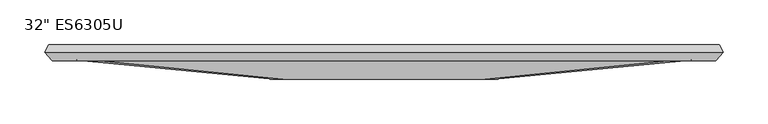
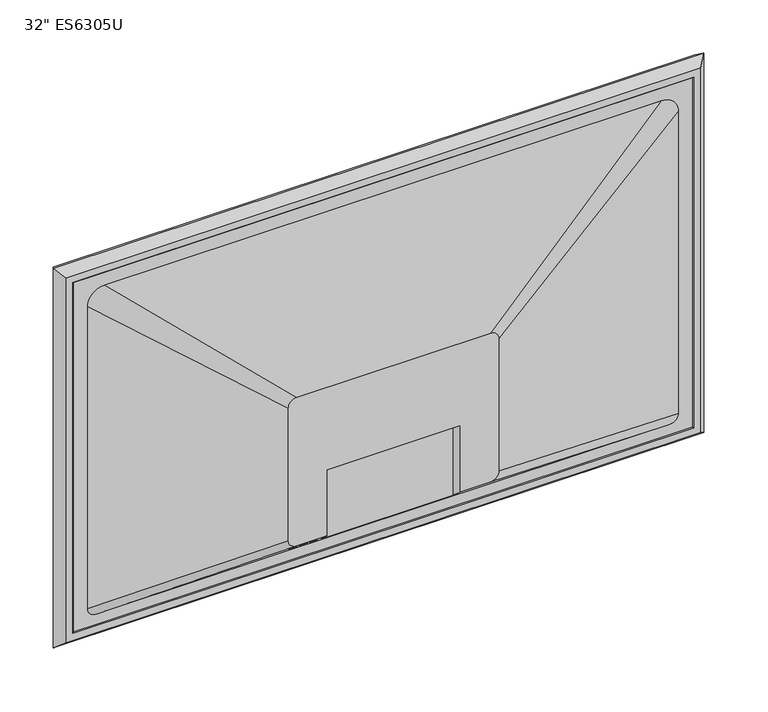
"""IFC4 building model written with IfcOpenShell, lengths in millimetres: proxy geometry."""

from ifc_helpers import new_model, si_unit, point, frame, origin, place, context, project, spatial, polyline, circle_curve, ellipse_curve, trimmed, outline, extrude, faceted_brep, source, transform, mapped, element, save
from ifc_brep_helpers import plane_surface, revolved_surface, extruded_surface, spline_surface, advanced_brep


def proxy_caca515e(model_context):
    return source(origin(), model_context, "Body", "SolidModel", [
        extrude(outline(polyline([(-245.0, 125.15), (495.0, 125.15), (495.0, 109.15), (-245.0, 109.15), (-245.0, 125.15)])), frame((0.0, 0.0, 1604.8), z_axis=(0.0, 0.0, 1.0), x_axis=(1.0, 0.0, 0.0)), (0.0, 0.0, 1.0), 448.0),
        advanced_brep(
        [(-205.0, 109.15, 2032.8), (455.0, 109.15, 2032.8), (475.0, 109.15, 2012.8), (475.0, 109.15, 1634.8), (465.0, 109.15, 1624.8), (-215.0, 109.15, 1624.8), (-225.0, 109.15, 1634.8), (-225.0, 109.15, 2012.8), (11.6666667, 87.15, 1828.8), (1.6666667, 87.15, 1818.8), (1.6666667, 87.15, 1654.8), (11.6666667, 87.15, 1644.8), (46.6666667, 87.15, 1644.8), (46.6666667, 87.15, 1726.8), (203.3333333, 87.15, 1726.8), (203.3333333, 87.15, 1644.8), (238.3333333, 87.15, 1644.8), (248.3333333, 87.15, 1654.8), (248.3333333, 87.15, 1818.8), (238.3333333, 87.15, 1828.8), (203.3333333, 103.15, 1630.2545455), (46.6666667, 103.15, 1630.2545455), (20.843372, 97.15, 1635.7090909), (28.843372, 97.15, 1635.7090909), (32.8393281, 97.15, 1635.7090909), (40.8393281, 97.15, 1635.7090909), (8.7618145, 97.15, 1635.7090909), (16.7618145, 97.15, 1635.7090909), (203.3333333, 103.15, 1726.8), (46.6666667, 103.15, 1726.8), (20.843372, 97.15, 1656.8), (24.843372, 97.15, 1656.8), (28.843372, 97.15, 1656.8), (32.8393281, 97.15, 1656.8), (36.8393281, 97.15, 1656.8), (40.8393281, 97.15, 1656.8), (8.7618145, 97.15, 1656.8), (12.7618145, 97.15, 1656.8), (16.7618145, 97.15, 1656.8)],
        [
            (0, 1),
            (1, 2, circle_curve(frame((455.0, 109.15, 2012.8), z_axis=(0.0, 1.0, 0.0), x_axis=(-1.0, 0.0, 0.0)), 20.0)),
            (2, 3),
            (3, 4, circle_curve(frame((465.0, 109.15, 1634.8), z_axis=(0.0, 1.0, 0.0), x_axis=(-1.0, 0.0, 0.0)), 10.0)),
            (4, 5),
            (5, 6, circle_curve(frame((-215.0, 109.15, 1634.8), z_axis=(0.0, 1.0, 0.0), x_axis=(-1.0, 0.0, 0.0)), 10.0)),
            (6, 7),
            (7, 0, circle_curve(frame((-205.0, 109.15, 2012.8), z_axis=(0.0, 1.0, 0.0), x_axis=(-1.0, 0.0, 0.0)), 20.0)),
            (8, 9, circle_curve(frame((11.6666667, 87.15, 1818.8), z_axis=(0.0, -1.0, 0.0), x_axis=(-1.0, 0.0, 0.0)), 10.0)),
            (9, 10),
            (10, 11, circle_curve(frame((11.6666667, 87.15, 1654.8), z_axis=(0.0, -1.0, 0.0), x_axis=(-1.0, 0.0, 0.0)), 10.0)),
            (11, 12),
            (12, 13),
            (13, 14),
            (14, 15),
            (15, 16),
            (16, 17, circle_curve(frame((238.3333333, 87.15, 1654.8), z_axis=(0.0, -1.0, 0.0), x_axis=(-1.0, 0.0, 0.0)), 10.0)),
            (17, 18),
            (18, 19, circle_curve(frame((238.3333333, 87.15, 1818.8), z_axis=(0.0, -1.0, 0.0), x_axis=(-1.0, 0.0, 0.0)), 10.0)),
            (19, 8),
            (0, 8),
            (19, 1),
            (18, 2),
            (17, 3),
            (16, 4),
            (15, 20),
            (20, 21),
            (21, 12),
            (11, 5),
            (22, 23, ellipse_curve(frame((24.843372, 97.15, 1635.7090909), z_axis=(0.0, 0.672672793996548, 0.7399400733957296), x_axis=(0.0, 0.7399400733957296, -0.6726727939965479)), 5.4058432, 4.0)),
            (23, 22, ellipse_curve(frame((24.843372, 97.15, 1635.7090909), z_axis=(0.0, 0.672672793996548, 0.7399400733957296), x_axis=(0.0, 0.7399400733957296, -0.6726727939965479)), 5.4058432, 4.0)),
            (24, 25, ellipse_curve(frame((36.8393281, 97.15, 1635.7090909), z_axis=(0.0, 0.672672793996548, 0.7399400733957296), x_axis=(0.0, 0.7399400733957296, -0.6726727939965479)), 5.4058432, 4.0)),
            (25, 24, ellipse_curve(frame((36.8393281, 97.15, 1635.7090909), z_axis=(0.0, 0.672672793996548, 0.7399400733957296), x_axis=(0.0, 0.7399400733957296, -0.6726727939965479)), 5.4058432, 4.0)),
            (26, 27, ellipse_curve(frame((12.7618145, 97.15, 1635.7090909), z_axis=(0.0, 0.672672793996548, 0.7399400733957296), x_axis=(0.0, 0.7399400733957296, -0.6726727939965479)), 5.4058432, 4.0)),
            (27, 26, ellipse_curve(frame((12.7618145, 97.15, 1635.7090909), z_axis=(0.0, 0.672672793996548, 0.7399400733957296), x_axis=(0.0, 0.7399400733957296, -0.6726727939965479)), 5.4058432, 4.0)),
            (10, 6),
            (9, 7),
            (28, 29),
            (29, 21),
            (20, 28),
            (28, 14),
            (13, 29),
            (30, 31),
            (31, 32),
            (32, 30, circle_curve(frame((24.843372, 97.15, 1656.8), z_axis=(0.0, 0.0, -1.0), x_axis=(1.0, 0.0, 0.0)), 4.0)),
            (30, 32, circle_curve(frame((24.843372, 97.15, 1656.8), z_axis=(0.0, 0.0, -1.0), x_axis=(1.0, 0.0, 0.0)), 4.0)),
            (32, 23),
            (22, 30),
            (33, 34),
            (34, 35),
            (35, 33, circle_curve(frame((36.8393281, 97.15, 1656.8), z_axis=(0.0, 0.0, -1.0), x_axis=(1.0, 0.0, 0.0)), 4.0)),
            (33, 35, circle_curve(frame((36.8393281, 97.15, 1656.8), z_axis=(0.0, 0.0, -1.0), x_axis=(1.0, 0.0, 0.0)), 4.0)),
            (35, 25),
            (24, 33),
            (36, 37),
            (37, 38),
            (38, 36, circle_curve(frame((12.7618145, 97.15, 1656.8), z_axis=(0.0, 0.0, -1.0), x_axis=(1.0, 0.0, 0.0)), 4.0)),
            (36, 38, circle_curve(frame((12.7618145, 97.15, 1656.8), z_axis=(0.0, 0.0, -1.0), x_axis=(1.0, 0.0, 0.0)), 4.0)),
            (38, 27),
            (26, 36),
        ],
        [
            plane_surface(frame((125.0, 109.15, 1826.3), z_axis=(0.0, 1.0, 0.0), x_axis=(1.0, 0.0, 0.0))),
            plane_surface(frame((125.0, 87.15, 1736.8), z_axis=(0.0, -1.0, 0.0), x_axis=(1.0, 0.0, 0.0))),
            plane_surface(frame((125.0, 87.15, 1828.8), z_axis=(0.0, -0.9942351648103037, 0.10722143934227057), x_axis=(1.0, 0.0, 0.0))),
            spline_surface(2, 1, [[(238.3333333, 87.15, 1828.8), (455.0, 109.15, 2032.8)], [(248.3333333, 87.15, 1828.8), (475.0, 109.15, 2032.8)], [(248.3333333, 87.15, 1818.8), (475.0, 109.15, 2012.8)]], [3, 3], [2, 2], [0.0, 1.0], [0.0, 1.0], weights=[[1.0, 1.0], [0.7071067811865476, 0.7071067811865476], [1.0, 1.0]]),
            plane_surface(frame((248.3333333, 87.15, 1736.8), z_axis=(0.09660486119908188, -0.9953228123542162, 0.0), x_axis=(0.0, 0.0, -1.0))),
            extruded_surface(trimmed(circle_curve(frame((238.3333333, 87.15, 1654.8), z_axis=(0.0, 1.0, 0.0), x_axis=(-1.0, 0.0, 0.0)), 10.0), [point((248.3333333, 87.15, 1654.8))], [point((238.3333333, 87.15, 1644.8))], True, "CARTESIAN"), (226.6666667, 22.0, -20.0), 228.60835022564004),
            plane_surface(frame((125.0, 87.15, 1644.8), z_axis=(0.0, -0.672672793996548, -0.7399400733957296), x_axis=(-1.0, 0.0, 0.0))),
            extruded_surface(trimmed(circle_curve(frame((11.6666667, 87.15, 1654.8), z_axis=(0.0, 1.0, 0.0), x_axis=(-1.0, 0.0, 0.0)), 10.0), [point((11.6666667, 87.15, 1644.8))], [point((1.6666667, 87.15, 1654.8))], True, "CARTESIAN"), (-226.6666667, 22.0, -20.0), 228.60835022564004),
            plane_surface(frame((1.6666667, 87.15, 1736.8), z_axis=(-0.09660486119908739, -0.9953228123542156, 0.0), x_axis=(0.0, 0.0, 1.0))),
            spline_surface(2, 1, [[(1.6666667, 87.15, 1818.8), (-225.0, 109.15, 2012.8)], [(1.6666667000000004, 87.15, 1828.8), (-225.0, 109.15, 2032.8)], [(11.6666667, 87.15, 1828.8), (-205.0, 109.15, 2032.8)]], [3, 3], [2, 2], [0.0, 1.0], [0.0, 1.0], weights=[[1.0, 1.0], [0.7071067811865476, 0.7071067811865476], [1.0, 1.0]]),
            plane_surface(frame((203.3333333, 103.15, 1726.8), z_axis=(0.0, -1.0, 0.0), x_axis=(1.0, 0.0, 0.0))),
            plane_surface(frame((46.6666667, 103.15, 1726.8), z_axis=(0.0, 0.0, -1.0), x_axis=(0.0, -1.0, 0.0))),
            plane_surface(frame((203.3333333, 103.15, 1726.8), z_axis=(-1.0, 0.0, 0.0), x_axis=(0.0, -1.0, 0.0))),
            plane_surface(frame((46.6666667, 103.15, 1604.8), z_axis=(1.0, 0.0, 0.0), x_axis=(0.0, -1.0, 0.0))),
            plane_surface(frame((24.843372, 97.15, 1656.8), z_axis=(0.0, 0.0, -1.0), x_axis=(1.0, 0.0, 0.0))),
            revolved_surface(polyline([(28.843372, 97.15, 1632.0727272507488), (28.843372, 97.15, 1656.8)]), (24.843372, 97.15, 1550.9439481), (0.0, 0.0, -1.0)),
            plane_surface(frame((36.8393281, 97.15, 1656.8), z_axis=(0.0, 0.0, -1.0), x_axis=(1.0, 0.0, 0.0))),
            revolved_surface(polyline([(40.8393281, 97.15, 1632.0727272507488), (40.8393281, 97.15, 1656.8)]), (36.8393281, 97.15, 1550.9439481), (0.0, 0.0, -1.0)),
            plane_surface(frame((12.7618145, 97.15, 1656.8), z_axis=(0.0, 0.0, -1.0), x_axis=(1.0, 0.0, 0.0))),
            revolved_surface(polyline([(16.7618145, 97.15, 1632.0727272507488), (16.7618145, 97.15, 1656.8)]), (12.7618145, 97.15, 1550.9439481), (0.0, 0.0, -1.0)),
        ],
        [
            (0, [[1, 2, 3, 4, 5, 6, 7, 8]]),
            (1, [[9, 10, 11, 12, 13, 14, 15, 16, 17, 18, 19, 20]]),
            (2, [[-1, 21, -20, 22]]),
            (3, [[-2, -22, -19, 23]]),
            (4, [[-3, -23, -18, 24]]),
            (5, [[-4, -24, -17, 25]]),
            (6, [[-5, -25, -16, 26, 27, 28, -12, 29], [30, 31], [32, 33], [34, 35]]),
            (7, [[-6, -29, -11, 36]]),
            (8, [[-7, -36, -10, 37]]),
            (9, [[-8, -37, -9, -21]]),
            (10, [[38, 39, -27, 40]]),
            (11, [[-38, 41, -14, 42]]),
            (12, [[-41, -40, -26, -15]]),
            (13, [[-42, -13, -28, -39]]),
            (14, [[43, 44, 45]]),
            (14, [[-43, 46, -44]]),
            (15, [[-45, 47, -30, 48]]),
            (15, [[-46, -48, -31, -47]]),
            (16, [[49, 50, 51]]),
            (16, [[-49, 52, -50]]),
            (17, [[-51, 53, -32, 54]]),
            (17, [[-52, -54, -33, -53]]),
            (18, [[55, 56, 57]]),
            (18, [[-55, 58, -56]]),
            (19, [[-57, 59, -34, 60]]),
            (19, [[-58, -60, -35, -59]]),
        ],
    ),
        faceted_brep([(-245.0, 125.15, 2052.8), (-245.0, 109.15, 2052.8), (-245.0, 109.15, 1604.8), (-245.0, 125.15, 1604.8), (-241.9959269, 126.15, 2049.7959269), (-240.6768394, 125.15, 2048.4768394), (-240.6768394, 125.15, 1609.1231606), (-241.9959269, 126.15, 1607.8040731), (-255.9259805, 117.6459377, 2063.7259805), (-251.0289147, 126.15, 2058.8289147), (-251.0289147, 126.15, 1598.7710853), (-255.9259805, 117.6459377, 1593.8740195), (-247.0701472, 108.15, 2054.8701472), (-247.0701472, 108.15, 1602.7298528), (-236.8560519, 109.15, 2044.6560519), (-238.5579741, 108.15, 2046.3579741), (-238.5579741, 108.15, 1611.2420259), (-236.8560519, 109.15, 1612.9439481), (495.0, 109.15, 1604.8), (495.0, 125.15, 1604.8), (490.6768394, 125.15, 1609.1231606), (491.9959269, 126.15, 1607.8040731), (501.0289147, 126.15, 1598.7710853), (505.9259805, 117.6459377, 1593.8740195), (497.0701472, 108.15, 1602.7298528), (488.5579741, 108.15, 1611.2420259), (486.8560519, 109.15, 1612.9439481), (495.0, 109.15, 2052.8), (495.0, 125.15, 2052.8), (490.6768394, 125.15, 2048.4768394), (491.9959269, 126.15, 2049.7959269), (501.0289147, 126.15, 2058.8289147), (505.9259805, 117.6459377, 2063.7259805), (497.0701472, 108.15, 2054.8701472), (488.5579741, 108.15, 2046.3579741), (486.8560519, 109.15, 2044.6560519)], [[[0, 1, 2, 3]], [[4, 5, 6, 7]], [[8, 9, 10, 11]], [[12, 8, 11, 13]], [[14, 15, 16, 17]], [[3, 2, 18, 19]], [[7, 6, 20, 21]], [[11, 10, 22, 23]], [[13, 11, 23, 24]], [[17, 16, 25, 26]], [[19, 18, 27, 28]], [[21, 20, 29, 30]], [[23, 22, 31, 32]], [[24, 23, 32, 33]], [[26, 25, 34, 35]], [[28, 27, 1, 0]], [[3, 19, 28, 0], [5, 29, 20, 6]], [[30, 29, 5, 4]], [[9, 31, 22, 10], [7, 21, 30, 4]], [[32, 31, 9, 8]], [[33, 32, 8, 12]], [[13, 24, 33, 12], [15, 34, 25, 16]], [[35, 34, 15, 14]], [[1, 27, 18, 2], [17, 26, 35, 14]]]),
    ])


if __name__ == "__main__":
    model = new_model("IFC4")
    model_context = context("Model", 3, world=origin())
    ifc_project = project(units=[si_unit("LENGTHUNIT", "METRE", prefix="MILLI")], contexts=[model_context])
    site = spatial("IfcSite", under=ifc_project)
    building = spatial("IfcBuilding", under=site)
    placement = place(None, origin())
    proxy_shape = proxy_caca515e(model_context)
    element("IfcBuildingElementProxy", 1, Name="32\" ES6305U", ObjectType="32\" ES6305U", at=placement, inside=building, context=model_context, shape_type="MappedRepresentation", body=[
        mapped(proxy_shape, transform((0.0, 0.0, 0.0), x_axis=(1.0, 0.0, 0.0), y_axis=(0.0, 1.0, 0.0), z_axis=(0.0, 0.0, 1.0))),
    ])
    save(model, "model.ifc")

# Revit data of these elements
# Type "32\" ES6305U"
#   URL = "http://www.samsung.com"
#   Model = "32ES6305U"
#   Manufacturer = "Samsung"
#   Description = "3D led smart tv, 6 series"
#   Width = 2' - 5.13386"
#   Placement height [instance default] = 5' - 6.92913"
#   Outputs inset = 0' - 0.3937"
#   Output size = 0' - 0.15748"
#   Inset corners = 0' - 0.3937"
#   Inset component exit = 0' - 1.77165"
#   Inset body = 0' - 0.7874"
#   Height = 1' - 5.6378"
#   Depth screen = 0' - 0.62992"
#   Depth frame edge = 0' - 0.03937"
#   Depth distance = 0' - 1.1811"
#   Depth body = 0' - 0.86614"
#   Screen material = TV Screen material
#   Frame material = TV Frame material
#   Body material = TV Body material
#   Default Elevation = 0
# Element 1 (IfcBuildingElementProxy, "32\" ES6305U")
#   Placement height = 6' - 0"
#   Materials on its faces: "TV Body material", "TV Frame material", "TV Screen material"
# Materials
#   "TV Screen material": class "Plastic", colour RGB 5 5 5, transparency 0, Description = "Plastic, generic, opaque black", Cost = 0
#   "TV Frame material": class "Metal", colour RGB 244 244 244, transparency 0, Cost = 0
#   "TV Body material": class "Plastic", colour RGB 31 31 31, transparency 0, Description = "Plastic, generic, opaque dark grey", Cost = 0
